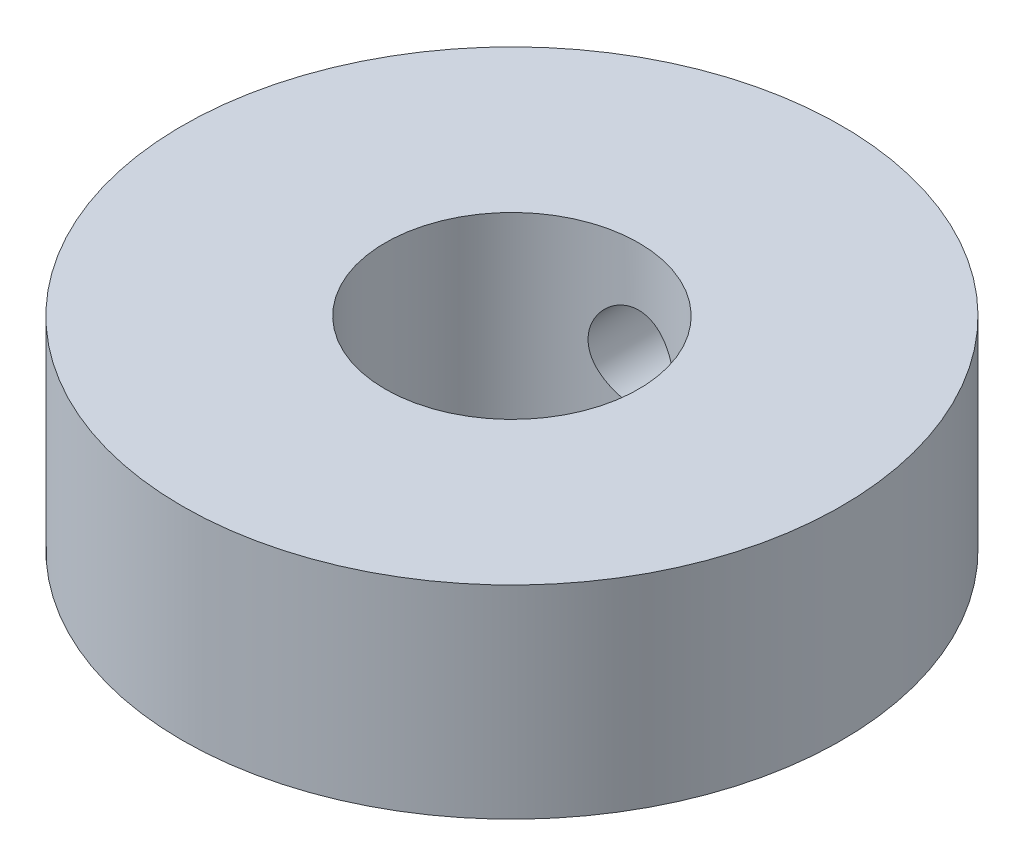
ISO-10303-21;
HEADER;
FILE_DESCRIPTION(('STEP AP214'),'2;1');
FILE_NAME('part.step','',(''),(''),'','','');
FILE_SCHEMA(('AUTOMOTIVE_DESIGN { 1 0 10303 214 1 1 1 1 }'));
ENDSEC;
DATA;
#1=APPLICATION_CONTEXT('core data for automotive mechanical design processes');
#2=APPLICATION_PROTOCOL_DEFINITION('international standard','automotive_design',2000,#1);
#3=PRODUCT_CONTEXT('',#1,'mechanical');
#4=PRODUCT('Part','Part','',(#3));
#5=PRODUCT_RELATED_PRODUCT_CATEGORY('part','',(#4));
#6=PRODUCT_DEFINITION_FORMATION('','',#4);
#7=PRODUCT_DEFINITION_CONTEXT('part definition',#1,'design');
#8=PRODUCT_DEFINITION('design','',#6,#7);
#9=PRODUCT_DEFINITION_SHAPE('','',#8);
#10=(LENGTH_UNIT() NAMED_UNIT(*) SI_UNIT(.MILLI.,.METRE.));
#11=(NAMED_UNIT(*) PLANE_ANGLE_UNIT() SI_UNIT($,.RADIAN.));
#12=(NAMED_UNIT(*) SI_UNIT($,.STERADIAN.) SOLID_ANGLE_UNIT());
#13=UNCERTAINTY_MEASURE_WITH_UNIT(LENGTH_MEASURE(1.E-05),#10,'distance_accuracy_value','');
#14=(GEOMETRIC_REPRESENTATION_CONTEXT(3) GLOBAL_UNCERTAINTY_ASSIGNED_CONTEXT((#13)) GLOBAL_UNIT_ASSIGNED_CONTEXT((#10,
#11,#12)) REPRESENTATION_CONTEXT('',''));
#15=CARTESIAN_POINT('',(0.,0.,0.));
#16=DIRECTION('',(0.,0.,1.));
#17=DIRECTION('',(1.,0.,0.));
#18=AXIS2_PLACEMENT_3D('',#15,#16,#17);
#19=CARTESIAN_POINT('',(0.,4.,0.));
#20=DIRECTION('',(0.,1.,0.));
#21=DIRECTION('',(0.,0.,1.));
#22=AXIS2_PLACEMENT_3D('',#19,#20,#21);
#23=PLANE('',#22);
#24=CARTESIAN_POINT('',(0.,4.,0.));
#25=DIRECTION('',(0.,1.,0.));
#26=DIRECTION('',(0.,0.,1.));
#27=AXIS2_PLACEMENT_3D('',#24,#25,#26);
#28=CIRCLE('',#27,6.5);
#29=CARTESIAN_POINT('',(0.,4.,6.5));
#30=VERTEX_POINT('',#29);
#31=EDGE_CURVE('E10',#30,#30,#28,.T.);
#32=ORIENTED_EDGE('',*,*,#31,.T.);
#33=EDGE_LOOP('',(#32));
#34=FACE_BOUND('',#33,.T.);
#35=CARTESIAN_POINT('',(0.,4.,0.));
#36=DIRECTION('',(0.,1.,0.));
#37=DIRECTION('',(0.,0.,1.));
#38=AXIS2_PLACEMENT_3D('',#35,#36,#37);
#39=CIRCLE('',#38,2.5);
#40=CARTESIAN_POINT('',(0.,4.,2.5));
#41=VERTEX_POINT('',#40);
#42=EDGE_CURVE('E61',#41,#41,#39,.T.);
#43=ORIENTED_EDGE('',*,*,#42,.F.);
#44=EDGE_LOOP('',(#43));
#45=FACE_BOUND('',#44,.T.);
#46=ADVANCED_FACE('F43',(#34,#45),#23,.T.);
#47=CARTESIAN_POINT('',(0.,0.,0.));
#48=DIRECTION('',(0.,1.,0.));
#49=DIRECTION('',(0.,0.,1.));
#50=AXIS2_PLACEMENT_3D('',#47,#48,#49);
#51=PLANE('',#50);
#52=CARTESIAN_POINT('',(0.,0.,0.));
#53=DIRECTION('',(0.,1.,0.));
#54=DIRECTION('',(0.,0.,1.));
#55=AXIS2_PLACEMENT_3D('',#52,#53,#54);
#56=CIRCLE('',#55,6.5);
#57=CARTESIAN_POINT('',(0.,0.,6.5));
#58=VERTEX_POINT('',#57);
#59=EDGE_CURVE('E60',#58,#58,#56,.T.);
#60=ORIENTED_EDGE('',*,*,#59,.F.);
#61=EDGE_LOOP('',(#60));
#62=FACE_BOUND('',#61,.T.);
#63=CARTESIAN_POINT('',(0.,0.,0.));
#64=DIRECTION('',(0.,1.,0.));
#65=DIRECTION('',(0.,0.,1.));
#66=AXIS2_PLACEMENT_3D('',#63,#64,#65);
#67=CIRCLE('',#66,2.5);
#68=CARTESIAN_POINT('',(0.,0.,2.5));
#69=VERTEX_POINT('',#68);
#70=EDGE_CURVE('E63',#69,#69,#67,.T.);
#71=ORIENTED_EDGE('',*,*,#70,.T.);
#72=EDGE_LOOP('',(#71));
#73=FACE_BOUND('',#72,.T.);
#74=ADVANCED_FACE('F84',(#62,#73),#51,.F.);
#75=CARTESIAN_POINT('',(0.,4.,0.));
#76=DIRECTION('',(0.,-1.,0.));
#77=DIRECTION('',(0.,0.,-1.));
#78=AXIS2_PLACEMENT_3D('',#75,#76,#77);
#79=CYLINDRICAL_SURFACE('',#78,6.5);
#80=CARTESIAN_POINT('',(0.,2.85,-6.5));
#81=CARTESIAN_POINT('',(-0.0475273119300373,2.84999799248828,-6.49999931236995));
#82=CARTESIAN_POINT('',(-0.0950838685352852,2.84600035816591,-6.49947323178086));
#83=CARTESIAN_POINT('',(-0.188872368165704,2.83011684021345,-6.49742520084858));
#84=CARTESIAN_POINT('',(-0.235102897000391,2.81822283933022,-6.49590222574721));
#85=CARTESIAN_POINT('',(-0.324868083813184,2.7869041035556,-6.49203188637918));
#86=CARTESIAN_POINT('',(-0.368404580616325,2.76748457249615,-6.48968509188108));
#87=CARTESIAN_POINT('',(-0.451592799552969,2.7216777075832,-6.48442776009261));
#88=CARTESIAN_POINT('',(-0.491245159131509,2.69529151969785,-6.48151731553985));
#89=CARTESIAN_POINT('',(-0.565785461247439,2.63613115202925,-6.47543781799476));
#90=CARTESIAN_POINT('',(-0.600646721904666,2.60332348431148,-6.47226746224011));
#91=CARTESIAN_POINT('',(-0.664385356510938,2.53232339768736,-6.46603589805202));
#92=CARTESIAN_POINT('',(-0.693262417465414,2.49413069730044,-6.46297469533459));
#93=CARTESIAN_POINT('',(-0.74431334689203,2.41326995922278,-6.4572952689164));
#94=CARTESIAN_POINT('',(-0.766462032006156,2.37058589399584,-6.45467872521815));
#95=CARTESIAN_POINT('',(-0.803266641578355,2.28206400552667,-6.45020220775352));
#96=CARTESIAN_POINT('',(-0.817922876539048,2.23622631306661,-6.44834220263528));
#97=CARTESIAN_POINT('',(-0.839245060342877,2.14297614512216,-6.44560189600989));
#98=CARTESIAN_POINT('',(-0.845956211853722,2.09557417116493,-6.44471605417936));
#99=CARTESIAN_POINT('',(-0.851337631414068,2.0003091413657,-6.44400745184395));
#100=CARTESIAN_POINT('',(-0.850008252370653,1.95244610585223,-6.44418464468137));
#101=CARTESIAN_POINT('',(-0.839383416745476,1.85793354974842,-6.44557702109154));
#102=CARTESIAN_POINT('',(-0.830137870368509,1.811278308926,-6.44678570114109));
#103=CARTESIAN_POINT('',(-0.804021074584761,1.72018722848242,-6.45009471801947));
#104=CARTESIAN_POINT('',(-0.787149657380238,1.67575143772138,-6.45219507446846));
#105=CARTESIAN_POINT('',(-0.746206767010475,1.59020626326385,-6.45705812107574));
#106=CARTESIAN_POINT('',(-0.72211372333688,1.54910732056856,-6.4598227905148));
#107=CARTESIAN_POINT('',(-0.667426908644924,1.47151694351829,-6.46570144773469));
#108=CARTESIAN_POINT('',(-0.636832812381057,1.43502573983264,-6.46881545298899));
#109=CARTESIAN_POINT('',(-0.569736309200595,1.36739708857793,-6.47507078642568));
#110=CARTESIAN_POINT('',(-0.533190905197018,1.33630228649931,-6.4782121429061));
#111=CARTESIAN_POINT('',(-0.455376896527025,1.28068155257026,-6.48414619584979));
#112=CARTESIAN_POINT('',(-0.414108279143427,1.25615563840706,-6.48693889137425));
#113=CARTESIAN_POINT('',(-0.327985545021085,1.21436838716425,-6.49186293139433));
#114=CARTESIAN_POINT('',(-0.283130052588049,1.1971098534394,-6.49399402059558));
#115=CARTESIAN_POINT('',(-0.191123614887421,1.1703818130707,-6.49735246309834));
#116=CARTESIAN_POINT('',(-0.143972787431609,1.16091190710848,-6.49857986273115));
#117=CARTESIAN_POINT('',(-0.0490827058108788,1.15008551807086,-6.49998658524286));
#118=CARTESIAN_POINT('',(-0.00135025940025587,1.14867031433475,-6.50017349332839));
#119=CARTESIAN_POINT('',(0.0936711479515367,1.15383834443808,-6.4994986892131));
#120=CARTESIAN_POINT('',(0.140960119225019,1.16042139146127,-6.49863700150446));
#121=CARTESIAN_POINT('',(0.233577960306399,1.18135026023174,-6.49596654168531));
#122=CARTESIAN_POINT('',(0.278913294107725,1.19566795181326,-6.49416120231276));
#123=CARTESIAN_POINT('',(0.366539538975663,1.2316303472019,-6.48980547358616));
#124=CARTESIAN_POINT('',(0.408830337795954,1.25327532098464,-6.48725505678));
#125=CARTESIAN_POINT('',(0.489428417687729,1.30341900138495,-6.48167440114856));
#126=CARTESIAN_POINT('',(0.527711980882102,1.3319555345954,-6.4786415468053));
#127=CARTESIAN_POINT('',(0.598967234536641,1.39501895679937,-6.47244311614296));
#128=CARTESIAN_POINT('',(0.631938693293378,1.42954610695535,-6.46927753404213));
#129=CARTESIAN_POINT('',(0.691843291628349,1.50386993358234,-6.46314688382087));
#130=CARTESIAN_POINT('',(0.718737409777831,1.5436981913656,-6.46018319234455));
#131=CARTESIAN_POINT('',(0.765453971337151,1.62734104705949,-6.45481490857007));
#132=CARTESIAN_POINT('',(0.78527656764822,1.67115555875319,-6.45241030418368));
#133=CARTESIAN_POINT('',(0.817224795407047,1.76140334255998,-6.44844196894699));
#134=CARTESIAN_POINT('',(0.829372110969365,1.80782882981979,-6.4468758710884));
#135=CARTESIAN_POINT('',(0.845694628529959,1.90208253157206,-6.44475519030191));
#136=CARTESIAN_POINT('',(0.849870239404839,1.94991067399319,-6.44420055549513));
#137=CARTESIAN_POINT('',(0.850122835656126,2.04522367056629,-6.44416720570299));
#138=CARTESIAN_POINT('',(0.846261133097074,2.0927083709792,-6.44468034527192));
#139=CARTESIAN_POINT('',(0.830678891126428,2.18634745705122,-6.44670717349693));
#140=CARTESIAN_POINT('',(0.818958353426524,2.23250184300008,-6.44822086193507));
#141=CARTESIAN_POINT('',(0.788010869452964,2.32216014144768,-6.45207564311972));
#142=CARTESIAN_POINT('',(0.768787167111572,2.36566518998194,-6.45441637825794));
#143=CARTESIAN_POINT('',(0.723385069356216,2.44884203326501,-6.45966206427547));
#144=CARTESIAN_POINT('',(0.697206554418634,2.48851376211941,-6.46256702485119));
#145=CARTESIAN_POINT('',(0.638411428341679,2.56321088075938,-6.46864036714318));
#146=CARTESIAN_POINT('',(0.605749169236973,2.59820019940238,-6.47181051866752));
#147=CARTESIAN_POINT('',(0.535009414588285,2.66222427410943,-6.4780415983337));
#148=CARTESIAN_POINT('',(0.496930648538757,2.69125762921894,-6.48110250063853));
#149=CARTESIAN_POINT('',(0.416255998760747,2.74264968738202,-6.48678438059768));
#150=CARTESIAN_POINT('',(0.373642000074418,2.76498014988817,-6.48940347710872));
#151=CARTESIAN_POINT('',(0.285257499923472,2.80213549893326,-6.49388776458797));
#152=CARTESIAN_POINT('',(0.239490454569184,2.81696845943889,-6.4957537661163));
#153=CARTESIAN_POINT('',(0.161244230967052,2.83519674337797,-6.49807688480155));
#154=CARTESIAN_POINT('',(0.129256406178424,2.84073987964473,-6.49879449916707));
#155=CARTESIAN_POINT('',(0.0648502577853982,2.84814217751771,-6.49975628940328));
#156=CARTESIAN_POINT('',(0.0324319377792675,2.85000136989644,-6.50000046922862));
#157=CARTESIAN_POINT('',(0.,2.85,-6.5));
#158=B_SPLINE_CURVE_WITH_KNOTS('',3,(#80,#81,#82,#83,#84,#85,#86,#87,#88,#89,#90,#91,#92,#93,
#94,#95,#96,#97,#98,#99,#100,#101,#102,#103,#104,#105,#106,#107,#108,#109,#110,#111,#112,#113,
#114,#115,#116,#117,#118,#119,#120,#121,#122,#123,#124,#125,#126,#127,#128,#129,#130,#131,#132,
#133,#134,#135,#136,#137,#138,#139,#140,#141,#142,#143,#144,#145,#146,#147,#148,#149,#150,#151,
#152,#153,#154,#155,#156,#157),.UNSPECIFIED.,.T.,.F.,(4,2,2,2,2,2,2,2,2,2,2,2,2,2,2,2,2,2,2,2,2,
2,2,2,2,2,2,2,2,2,2,2,2,2,2,2,2,2,4),(0.,0.142463462525733,0.285073600902839,0.427585301196982,
0.57007357386517,0.713325732172383,0.856585381178341,1.000374805454,1.14415827031556,
1.28711970254374,1.43007486009443,1.57213528912614,1.71419884417195,1.856691035145,
1.99919035663422,2.14276903568952,2.28634810133738,2.4299825012501,2.57360953665222,
2.71618814287226,2.85876341892822,3.0008236193046,3.14288905449594,3.28575273104674,
3.42862263734086,3.57238534735202,3.71614494872143,3.85949656443053,4.00284082729618,
4.14509560786373,4.28735035744755,4.42954367235129,4.57173943111082,4.71497427359934,
4.85824276908101,5.00210667226393,5.14581531835641,5.24303109934419,5.34024606827101),.UNSPECIFIED.);
#159=CARTESIAN_POINT('',(0.,2.85,-6.5));
#160=VERTEX_POINT('',#159);
#161=EDGE_CURVE('E70',#160,#160,#158,.T.);
#162=ORIENTED_EDGE('',*,*,#161,.T.);
#163=EDGE_LOOP('',(#162));
#164=FACE_BOUND('',#163,.T.);
#165=ORIENTED_EDGE('',*,*,#31,.F.);
#166=EDGE_LOOP('',(#165));
#167=FACE_BOUND('',#166,.T.);
#168=ORIENTED_EDGE('',*,*,#59,.T.);
#169=EDGE_LOOP('',(#168));
#170=FACE_BOUND('',#169,.T.);
#171=ADVANCED_FACE('F44',(#164,#167,#170),#79,.T.);
#172=CARTESIAN_POINT('',(0.,4.,0.));
#173=DIRECTION('',(0.,-1.,0.));
#174=DIRECTION('',(0.,0.,-1.));
#175=AXIS2_PLACEMENT_3D('',#172,#173,#174);
#176=CYLINDRICAL_SURFACE('',#175,2.5);
#177=CARTESIAN_POINT('',(0.,2.85,-2.5));
#178=CARTESIAN_POINT('',(-0.0463258633171595,2.85000040660683,-2.5000002698726));
#179=CARTESIAN_POINT('',(-0.0926489204520312,2.84620053340924,-2.4987005737574));
#180=CARTESIAN_POINT('',(-0.183927439746679,2.83115021018598,-2.49364411759606));
#181=CARTESIAN_POINT('',(-0.228882813989826,2.81989928224976,-2.48988719994395));
#182=CARTESIAN_POINT('',(-0.316096879446529,2.79037930760111,-2.48032377466595));
#183=CARTESIAN_POINT('',(-0.358360043646003,2.7721222756574,-2.47452077723828));
#184=CARTESIAN_POINT('',(-0.439224077997479,2.72916369623689,-2.4614552731555));
#185=CARTESIAN_POINT('',(-0.477824178583485,2.70446079862998,-2.45419246080558));
#186=CARTESIAN_POINT('',(-0.551650523889469,2.64838213837963,-2.43867820570341));
#187=CARTESIAN_POINT('',(-0.586727376243688,2.61681648842439,-2.43040239451419));
#188=CARTESIAN_POINT('',(-0.651204667601688,2.54831194018363,-2.4139266876053));
#189=CARTESIAN_POINT('',(-0.680603788011975,2.51137179721281,-2.40572680994034));
#190=CARTESIAN_POINT('',(-0.733758381552362,2.43180454412124,-2.39006097264164));
#191=CARTESIAN_POINT('',(-0.757317108727101,2.38903961410482,-2.3826245722385));
#192=CARTESIAN_POINT('',(-0.796843710361144,2.29986106787469,-2.36969950654034));
#193=CARTESIAN_POINT('',(-0.812814008539866,2.25344862219259,-2.36421021948586));
#194=CARTESIAN_POINT('',(-0.836145431711188,2.15999509345478,-2.35605808278384));
#195=CARTESIAN_POINT('',(-0.84378735430839,2.11303237203158,-2.35330334512171));
#196=CARTESIAN_POINT('',(-0.851123009937607,2.01841669866582,-2.35066081888085));
#197=CARTESIAN_POINT('',(-0.850819317817387,1.97076397532753,-2.35077210154233));
#198=CARTESIAN_POINT('',(-0.842489868052584,1.87854101084113,-2.35376871343028));
#199=CARTESIAN_POINT('',(-0.834833884085795,1.83393229925284,-2.3565212015213));
#200=CARTESIAN_POINT('',(-0.812621633057355,1.74667490251601,-2.36427219830348));
#201=CARTESIAN_POINT('',(-0.798064508460424,1.70402646167325,-2.36927098611566));
#202=CARTESIAN_POINT('',(-0.762227306076265,1.62107352575003,-2.38104368569454));
#203=CARTESIAN_POINT('',(-0.740839801464803,1.58081959428648,-2.38784564505742));
#204=CARTESIAN_POINT('',(-0.69202354799802,1.5043565852273,-2.40244689518169));
#205=CARTESIAN_POINT('',(-0.664592998280718,1.46814871824027,-2.41024648295086));
#206=CARTESIAN_POINT('',(-0.602706248429934,1.39873229794268,-2.42648332831841));
#207=CARTESIAN_POINT('',(-0.567948790070821,1.36579447129138,-2.43493218082336));
#208=CARTESIAN_POINT('',(-0.49330035398348,1.30614293445113,-2.45114500377937));
#209=CARTESIAN_POINT('',(-0.453408843955487,1.27942987045544,-2.45890890307342));
#210=CARTESIAN_POINT('',(-0.369032873506826,1.23275634400495,-2.4729862471248));
#211=CARTESIAN_POINT('',(-0.32450388937437,1.21287108764486,-2.47928330633144));
#212=CARTESIAN_POINT('',(-0.232467106988595,1.18095852578253,-2.48959818880685));
#213=CARTESIAN_POINT('',(-0.184960393985483,1.16892837548357,-2.49361683715291));
#214=CARTESIAN_POINT('',(-0.090606561389721,1.15355333040445,-2.49878413767634));
#215=CARTESIAN_POINT('',(-0.043825554473044,1.14984281670371,-2.50005351932376));
#216=CARTESIAN_POINT('',(0.0497016468544445,1.15016733866702,-2.49994302787298));
#217=CARTESIAN_POINT('',(0.0964478459535919,1.1542010068229,-2.49856362251145));
#218=CARTESIAN_POINT('',(0.187097411183407,1.16961164679269,-2.49339029178394));
#219=CARTESIAN_POINT('',(0.23104399839399,1.18076190915309,-2.48967095875153));
#220=CARTESIAN_POINT('',(0.3164231429474,1.20980349156516,-2.48026663942839));
#221=CARTESIAN_POINT('',(0.357855376664244,1.22769567725171,-2.47458140073128));
#222=CARTESIAN_POINT('',(0.438271708726932,1.27024469075598,-2.46162999094866));
#223=CARTESIAN_POINT('',(0.477160102287992,1.2950703781274,-2.45432544235829));
#224=CARTESIAN_POINT('',(0.550336613102922,1.3505845769571,-2.43896082572603));
#225=CARTESIAN_POINT('',(0.584623270006919,1.38127494210262,-2.43090051921814));
#226=CARTESIAN_POINT('',(0.64931470257648,1.44936551330125,-2.41444772266588));
#227=CARTESIAN_POINT('',(0.679458657687896,1.48701469758571,-2.40605758371095));
#228=CARTESIAN_POINT('',(0.733036041745385,1.56701557559396,-2.39028046986892));
#229=CARTESIAN_POINT('',(0.756469348659538,1.60936735481415,-2.38289351322579));
#230=CARTESIAN_POINT('',(0.795867339083949,1.69763133607519,-2.3700267261547));
#231=CARTESIAN_POINT('',(0.811841507809274,1.74353892932578,-2.36454447594177));
#232=CARTESIAN_POINT('',(0.835755258120592,1.83762351353113,-2.35619962971029));
#233=CARTESIAN_POINT('',(0.843698654647643,1.88579941555367,-2.35333578990298));
#234=CARTESIAN_POINT('',(0.851020580432781,1.98028505400886,-2.35069725021723));
#235=CARTESIAN_POINT('',(0.850833768663468,2.02655709009667,-2.35076577610729));
#236=CARTESIAN_POINT('',(0.842977076196028,2.11837331350791,-2.35359441824177));
#237=CARTESIAN_POINT('',(0.835307675963531,2.16391754737352,-2.35635436166716));
#238=CARTESIAN_POINT('',(0.813016339031805,2.25204973399144,-2.36413587826503));
#239=CARTESIAN_POINT('',(0.798540669099527,2.29467922773508,-2.36910975930576));
#240=CARTESIAN_POINT('',(0.763167585454484,2.37693623379672,-2.38073943073194));
#241=CARTESIAN_POINT('',(0.74226871096473,2.41656306068466,-2.38739560364607));
#242=CARTESIAN_POINT('',(0.693544147047599,2.49362674097299,-2.40201380937306));
#243=CARTESIAN_POINT('',(0.665448697744606,2.53088437489126,-2.41002117941802));
#244=CARTESIAN_POINT('',(0.603578512030883,2.60029639820325,-2.42625527464081));
#245=CARTESIAN_POINT('',(0.569802139666918,2.63244931237516,-2.43448206242921));
#246=CARTESIAN_POINT('',(0.495860317584488,2.69207592901612,-2.45063468659226));
#247=CARTESIAN_POINT('',(0.455489089524437,2.71930251060318,-2.45853419137891));
#248=CARTESIAN_POINT('',(0.370479539684275,2.76655610452008,-2.47277150035442));
#249=CARTESIAN_POINT('',(0.325842107342673,2.78658461341127,-2.47910962908485));
#250=CARTESIAN_POINT('',(0.23499710820746,2.81823990931925,-2.48933696610399));
#251=CARTESIAN_POINT('',(0.188882674896089,2.83011046978427,-2.49329673714849));
#252=CARTESIAN_POINT('',(0.0951775378488083,2.84598910854748,-2.49862772115815));
#253=CARTESIAN_POINT('',(0.0475872883823168,2.84999958232152,-2.49999972277893));
#254=CARTESIAN_POINT('',(0.,2.85,-2.5));
#255=B_SPLINE_CURVE_WITH_KNOTS('',3,(#177,#178,#179,#180,#181,#182,#183,#184,#185,#186,#187,
#188,#189,#190,#191,#192,#193,#194,#195,#196,#197,#198,#199,#200,#201,#202,#203,#204,#205,#206,
#207,#208,#209,#210,#211,#212,#213,#214,#215,#216,#217,#218,#219,#220,#221,#222,#223,#224,#225,
#226,#227,#228,#229,#230,#231,#232,#233,#234,#235,#236,#237,#238,#239,#240,#241,#242,#243,#244,
#245,#246,#247,#248,#249,#250,#251,#252,#253,#254),.UNSPECIFIED.,.T.,.F.,(4,2,2,2,2,2,2,2,2,2,2,
2,2,2,2,2,2,2,2,2,2,2,2,2,2,2,2,2,2,2,2,2,2,2,2,2,2,2,4),(0.,0.138802406227104,
0.277613716101145,0.416188034615628,0.554791401788676,0.697875099489832,0.840991987019438,
0.988421253571527,1.13580339999263,1.27804604996183,1.42024260549472,1.5556428066994,
1.6910598371359,1.82872125648959,1.9664237553603,2.11162544164018,2.25684219461353,
2.4036106825306,2.550325987406,2.69045562996828,2.83056052998071,2.96641094415789,
3.10227880690895,3.24179771358495,3.38136079207934,3.52753496246494,3.67371179083256,
3.81970222768387,3.96562328055048,4.10375316783866,4.24187418623126,4.37715390367015,
4.51246440946465,4.65387390477818,4.7953241921703,4.94259759301293,5.08984035629915,
5.23246574150158,5.37504765277796),.UNSPECIFIED.);
#256=CARTESIAN_POINT('',(0.,2.85,-2.5));
#257=VERTEX_POINT('',#256);
#258=EDGE_CURVE('E48',#257,#257,#255,.T.);
#259=ORIENTED_EDGE('',*,*,#258,.F.);
#260=EDGE_LOOP('',(#259));
#261=FACE_BOUND('',#260,.T.);
#262=ORIENTED_EDGE('',*,*,#42,.T.);
#263=EDGE_LOOP('',(#262));
#264=FACE_BOUND('',#263,.T.);
#265=ORIENTED_EDGE('',*,*,#70,.F.);
#266=EDGE_LOOP('',(#265));
#267=FACE_BOUND('',#266,.T.);
#268=ADVANCED_FACE('F76',(#261,#264,#267),#176,.F.);
#269=CARTESIAN_POINT('',(0.,2.,-7.));
#270=DIRECTION('',(0.,0.,1.));
#271=DIRECTION('',(1.,0.,0.));
#272=AXIS2_PLACEMENT_3D('',#269,#270,#271);
#273=CYLINDRICAL_SURFACE('',#272,0.85);
#274=ORIENTED_EDGE('',*,*,#258,.T.);
#275=EDGE_LOOP('',(#274));
#276=FACE_BOUND('',#275,.T.);
#277=ORIENTED_EDGE('',*,*,#161,.F.);
#278=EDGE_LOOP('',(#277));
#279=FACE_BOUND('',#278,.T.);
#280=ADVANCED_FACE('F74',(#276,#279),#273,.F.);
#281=CLOSED_SHELL('',(#46,#74,#171,#268,#280));
#282=MANIFOLD_SOLID_BREP('B2',#281);
#283=ADVANCED_BREP_SHAPE_REPRESENTATION('',(#18,#282),#14);
#284=SHAPE_DEFINITION_REPRESENTATION(#9,#283);
ENDSEC;
END-ISO-10303-21;
